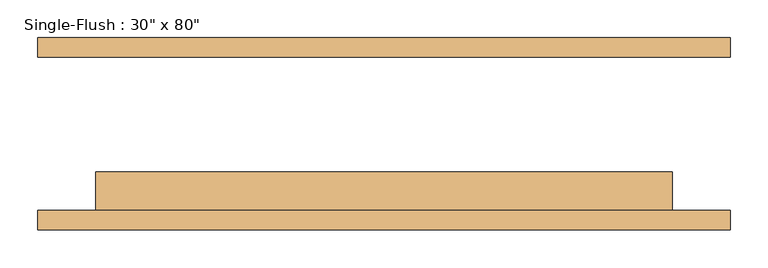
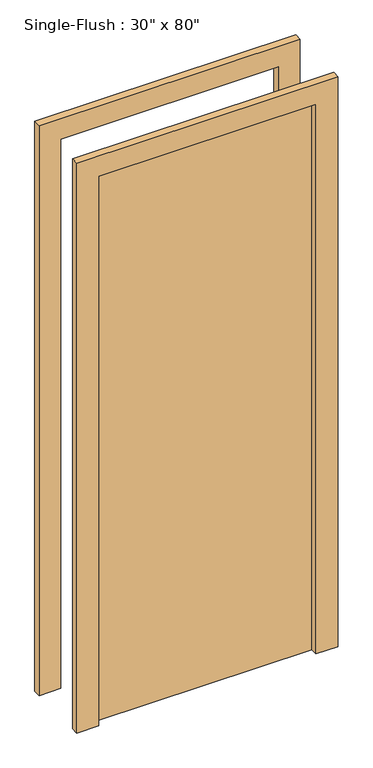
"""IFC4 building model written with IfcOpenShell, lengths in millimetres: door geometry."""

from ifc_helpers import new_model, si_unit, frame, origin, origin_with_axes, place, context, project, spatial, polyline, outline, extrude, source, transform, mapped, element, save


def door_53b1b562(model_context):
    return source(origin(), model_context, "Body", "SweptSolid", [
        extrude(outline(polyline([(2108.2, -457.2), (0.0, -457.2), (0.0, -381.0), (2032.0, -381.0), (2032.0, 381.0), (0.0, 381.0), (0.0, 457.2), (2108.2, 457.2), (2108.2, -457.2)])), frame((0.0, -127.0, 0.0), z_axis=(0.0, 1.0, 0.0), x_axis=(0.0, 0.0, 1.0)), (0.0, 0.0, 1.0), 25.4),
        extrude(outline(polyline([(2108.2, 457.2), (2108.2, -457.2), (0.0, -457.2), (0.0, -381.0), (2032.0, -381.0), (2032.0, 381.0), (0.0, 381.0), (0.0, 457.2), (2108.2, 457.2)])), frame((0.0, 101.6, 0.0), z_axis=(0.0, 1.0, 0.0), x_axis=(0.0, 0.0, 1.0)), (0.0, 0.0, 1.0), 25.4),
        extrude(outline(polyline([(381.0, -50.8), (381.0, -101.6), (-381.0, -101.6), (-381.0, -50.8), (381.0, -50.8)])), origin_with_axes(), (0.0, 0.0, 1.0), 2032.0),
    ])


if __name__ == "__main__":
    model = new_model("IFC4")
    model_context = context("Model", 3, world=origin())
    ifc_project = project(units=[si_unit("LENGTHUNIT", "METRE", prefix="MILLI")], contexts=[model_context])
    site = spatial("IfcSite", under=ifc_project)
    building = spatial("IfcBuilding", under=site)
    placement = place(None, origin())
    door_shape = door_53b1b562(model_context)
    element("IfcDoor", 1, ObjectType="Single-Flush : 30\" x 80\"", at=placement, inside=building, context=model_context, shape_type="MappedRepresentation", body=[
        mapped(door_shape, transform((0.0, 0.0, 0.0), x_axis=(1.0, 0.0, 0.0), y_axis=(0.0, 1.0, 0.0), z_axis=(0.0, 0.0, 1.0))),
    ])
    save(model, "model.ifc")

# Revit data of these elements
# Type "Single-Flush : 30\" x 80\""
#   Type Mark = "5"
#   Construction Type Id = "MDOOR"
#   Assembly Code = "C1020"
#   Analytic Construction = "Metal"
#   Thickness = 0' - 2"
#   Heat Transfer Coefficient (U) = 0.651978 BTU/(h·ft²·°F)
#   Height = 6' - 8"
#   Trim Projection Ext = 0' - 1"
#   Trim Projection Int = 0' - 1"
#   Trim Width = 0' - 3"
#   Width = 2' - 6"
#   Define Thermal Properties by = 1
#   Define Thermal Properties by = 1
#   Door Material = Door - Panel
#   Frame Material = Door - Frame
#   Visual Light Transmittance = 0
#   Solar Heat Gain Coefficient = 0
#   Function = (empty or 0)
#   Wall Closure = (empty or 0)
# Element 1 (IfcDoor, "Single-Flush : 30\" x 80\"")
#   Materials on its faces: "Door - Frame", "Door - Panel"
# Materials
#   "Door - Panel": class "Wood", colour RGB 210 159 95, transparency 0, Cost = 0
#   "Door - Frame": colour RGB 118 70 51, transparency 0, Cost = 0
